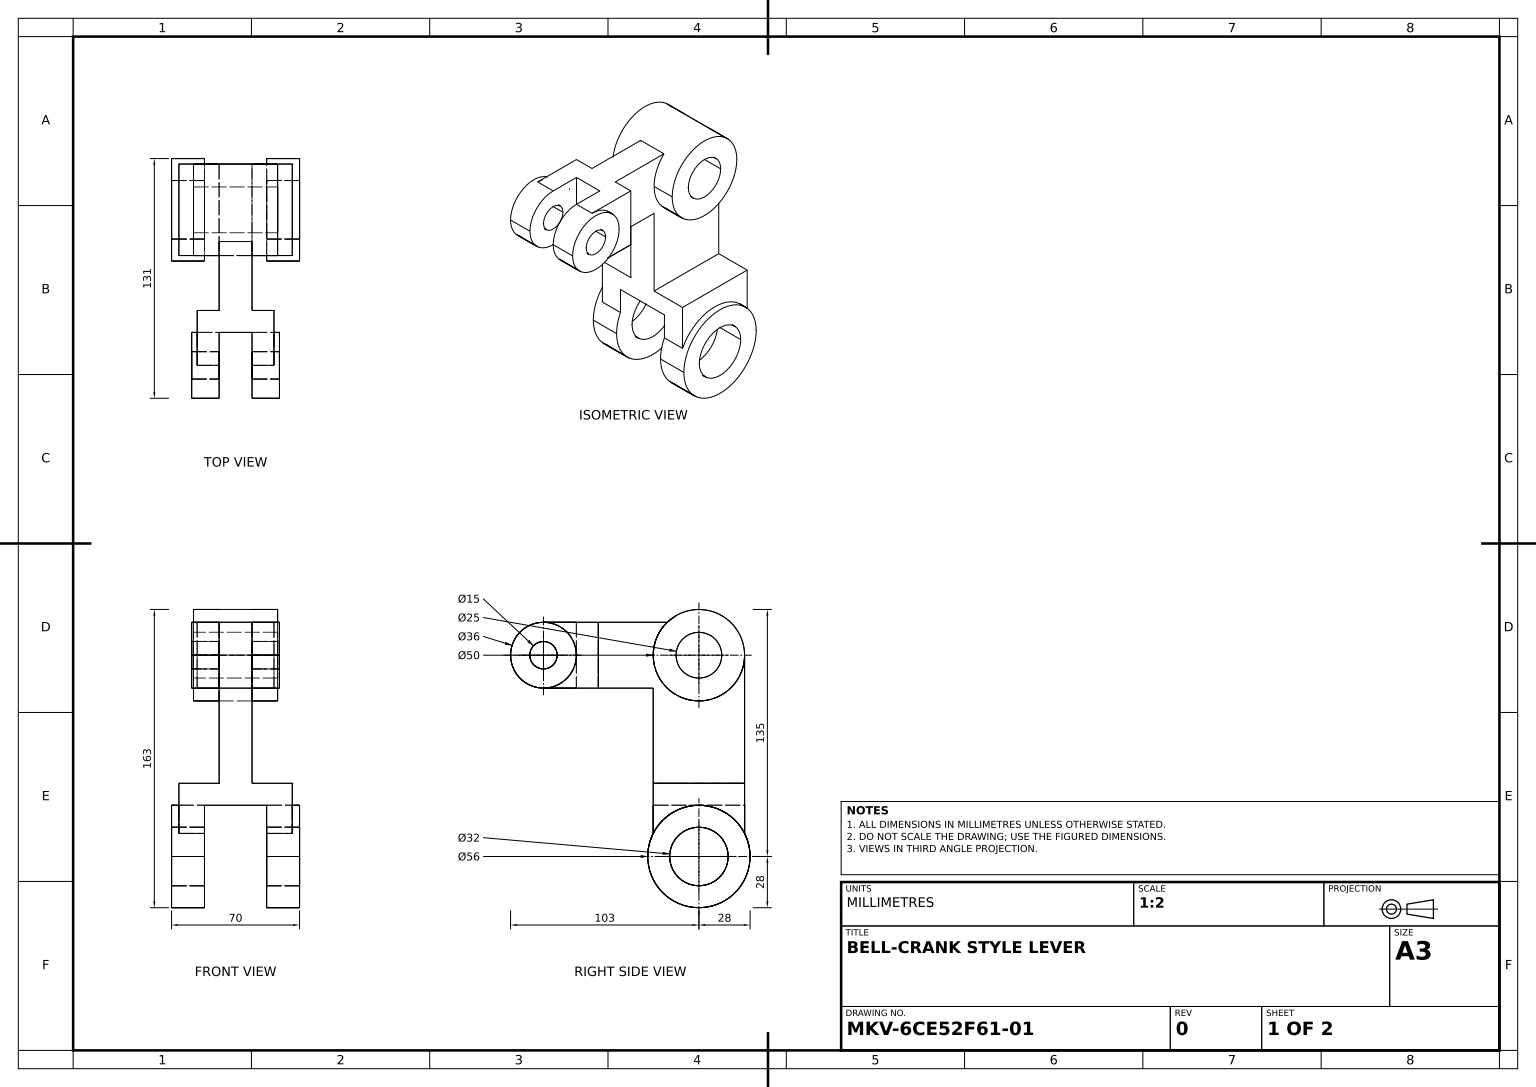
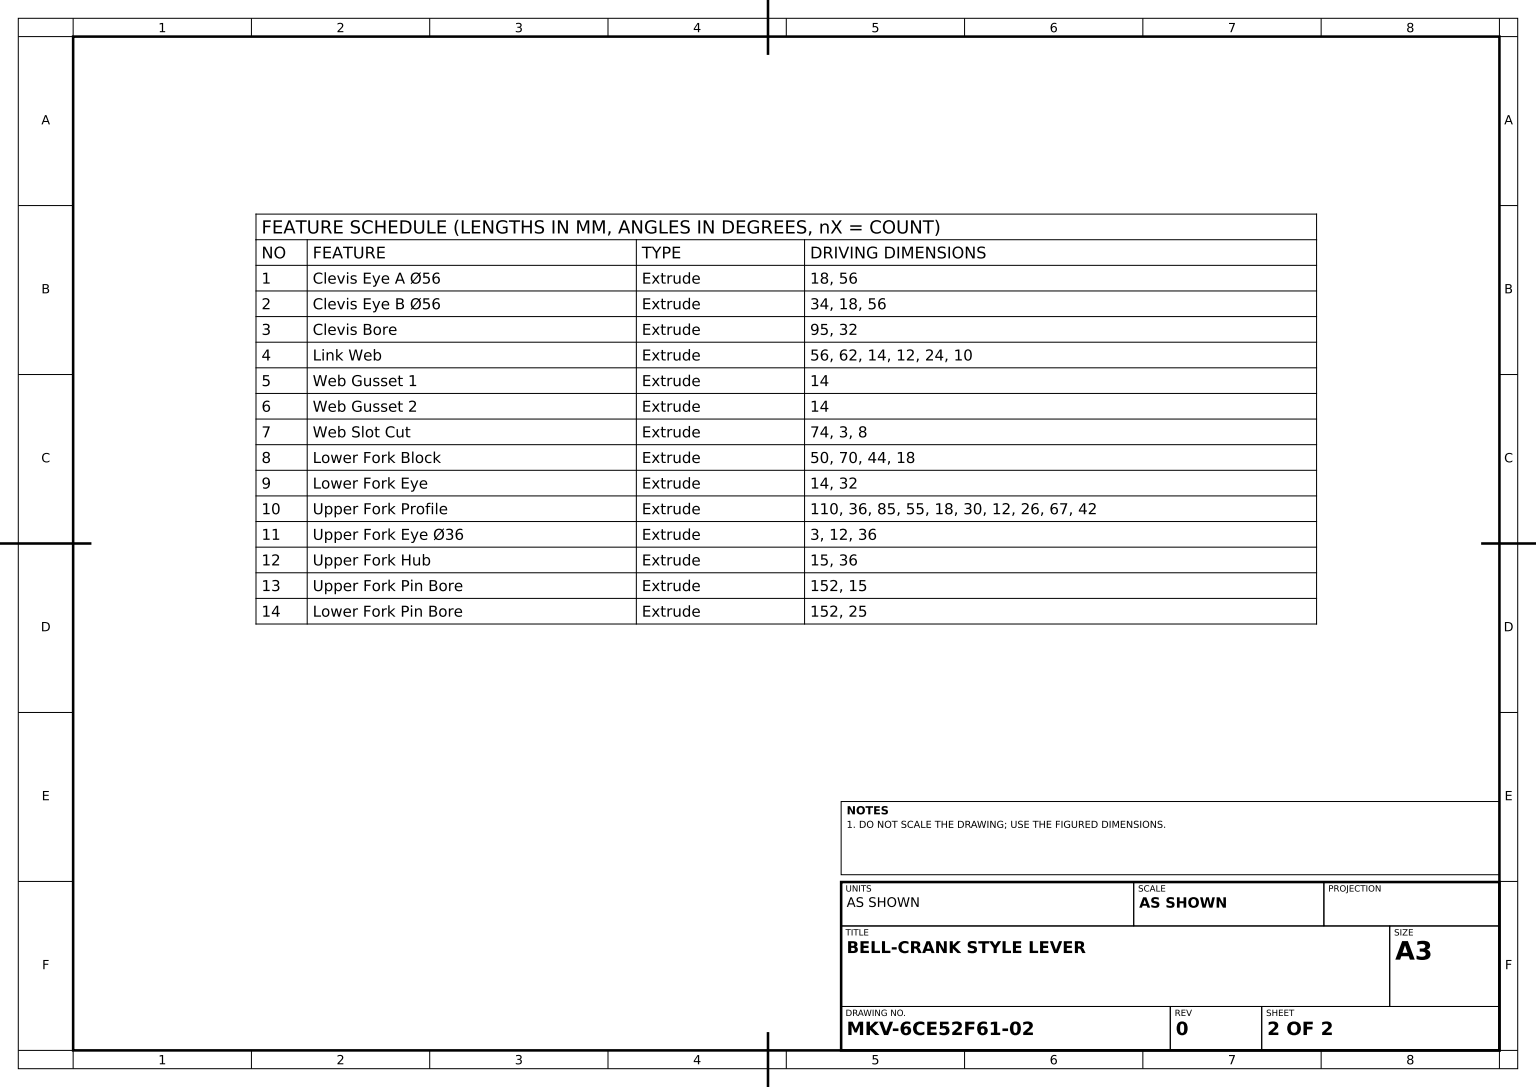
SolidWorks part; units mm, degrees
material "Plain Carbon Steel"
ref_plane "Front Plane" through (0, 0, 0) normal (0, 0, 1) x (1, 0, 0)
ref_plane "Top Plane" through (0, 0, 0) normal (0, 1, 0) x (1, 0, 0)
ref_plane "Right Plane" through (0, 0, 0) normal (1, 0, 0) x (0, 0, -1)
sketch "Clevis Eye A Sketch" plane through (0, 0, 0) normal (1, 0, 0) x (0, 0, -1)
  circle A0 centre (0, 0) radius 28
  dimension "D1" = 56
extrude "Clevis Eye A Ø56" add sketch "Clevis Eye A Sketch" against normal blind 18
ref_plane "Clevis Eye B Plane" through (-52, 0, 0) normal (-1, 0, 0) x (0, 0, 1)
sketch "Clevis Eye B Sketch" plane through (-52, 0, 0) normal (-1, 0, 0) x (0, 0, 1)
  circle A0 centre (0, 0) radius 28
  dimension "D1" = 56
extrude "Clevis Eye B Ø56" add sketch "Clevis Eye B Sketch" along normal blind 18 separate body
sketch "Clevis Bore Sketch" plane through (0, 0, 0) normal (1, 0, 0) x (0, 0, -1)
  circle A0 centre (0, 0) radius 16
  dimension "D1" = 32
extrude "Clevis Bore" cut sketch "Clevis Bore Sketch" against normal blind 95
sketch "Link Web Sketch" plane through (0, 0, 0) normal (0, 0, 1) x (1, 0, 0)
  line L0 (-66, 16) -> (-52, 16)
  line L3 (-4, 40) -> (-66, 40)
  line L6 (-52, -28) -> (-52, 28) construction
  line L7 (-52, 26) -> (-52, 28)
  line L8 (-52, 28) -> (-18, 28)
  line L9 (-18, 28) -> (-18, 26)
  line L10 (-18, 28) -> (-18, -28) construction
  line L12 (-66, 40) -> (-66, 16)
  line L13 (-52, 16) -> (-52, 28)
  line L14 (-4, 40) -> (-4, 16)
  line L15 (-4, 16) -> (-18, 16)
  line L16 (-18, 16) -> (-18, 28)
  dimension "D1" = 62
  dimension "D2" = 14
  dimension "D3" = 12
  dimension "D4" = 24
  dimension "D5" = 10
extrude "Link Web" add sketch "Link Web Sketch" along normal mid plane 56 contours L16 L15 L14 L3 L12 L0 L13 L7 L8 L9
sketch "Web Gusset 1 Sketch" plane through (-4, 0, 0) normal (1, 0, 0) x (0, 0, -1)
  line L0 (-28, 16) -> (-28, 0)
  line L1 (28, 16) -> (28, 0)
  line L2 (-28, 16) -> (-22.9783, 16)
  line L3 (22.9783, 16) -> (28, 16)
  circle A0 centre (0, 0) radius 28 construction
  arc A1 (28, 0) -> (22.9783, 16) centre (0, 0) ccw
  arc A2 (-22.9783, 16) -> (-28, 0) centre (0, 0) ccw
extrude "Web Gusset 1" add sketch "Web Gusset 1 Sketch" against normal blind 14
sketch "Web Gusset 2 Sketch" plane through (-66, 0, 0) normal (-1, 0, 0) x (0, 0, 1)
  line L0 (28, 16) -> (28, 0)
  line L1 (-28, 0) -> (-28, 16)
  line L2 (-28, 16) -> (-22.9783, 16)
  line L3 (28, 16) -> (22.9783, 16)
  circle A0 centre (0, 0) radius 28 construction
  arc A3 (28, 0) -> (22.9783, 16) centre (0, 0) ccw
  arc A4 (-22.9783, 16) -> (-28, 0) centre (0, 0) ccw
extrude "Web Gusset 2" add sketch "Web Gusset 2 Sketch" against normal blind 14
sketch "Web Slot Sketch" plane through (-4, 0, 0) normal (1, 0, 0) x (0, 0, -1)
  line L0 (0, 40) -> (25, 40)
  line L1 (-28, 40) -> (28, 40) construction
  line L2 (25, 40) -> (25, 8)
  line L3 (25, 8) -> (-25, 8)
  line L4 (-25, 8) -> (-25, 40)
  line L5 (-25, 40) -> (0, 40)
  line L6 (25, 40) -> (28, 40)
  line L7 (28, 40) -> (28, 0)
  line L8 (-28, 40) -> (-28, 0)
  line L9 (-28, 40) -> (-28, 0) construction
  arc A0 (28, 0) -> (25, 12.6095) centre (0, 0) ccw
  arc A1 (-25, 12.6095) -> (-28, 0) centre (0, 0) ccw
  line M7 (-28, 40) -> (-28, 0)
  arc M8 (-28, 0) -> (28, 0) centre (0, 0) cw
  line M9 (28, 0) -> (28, 40)
  line M10 (28, 40) -> (-28, 40)
  dimension "D1" = 3
  dimension "D2" = 8
extrude "Web Slot Cut" cut sketch "Web Slot Sketch" against normal blind 74 contours L4 M8 M10 M7 | L2 M10 M8 M9
sketch "Lower Fork Block Sketch" plane through (0, 0, 25) normal (0, 0, 1) x (1, 0, 0)
  line L0 (-44, 40) -> (-26, 40)
  line L1 (-66, 40) -> (-4, 40) construction
  line L2 (-44, 40) -> (-44, 110)
  line L3 (-44, 110) -> (-26, 110)
  line L4 (-26, 110) -> (-26, 40)
  dimension "D1" = 70
  dimension "D2" = 44
  dimension "D3" = 18
extrude "Lower Fork Block" add sketch "Lower Fork Block Sketch" against normal blind 50
sketch "Lower Fork Eye Sketch" plane through (-44, 0, 0) normal (-1, 0, 0) x (0, 0, 1)
  line L0 (-25, 110) -> (25, 110) construction
  circle A0 centre (0, 110) radius 25
extrude "Lower Fork Eye" add sketch "Lower Fork Eye Sketch" along normal blind 14 and the other way blind 32
ref_plane "Fork End Plane" through (0, 110, 0) normal (0, 1, 0) x (1, 0, 0)
sketch "Upper Fork Profile Sketch" plane through (0, 110, 0) normal (0, 1, 0) x (1, 0, 0)
  line L1 (-26, -55) -> (-14, -55)
  line L14 (-26, 0) -> (-26, -55)
  line L16 (-44, -55) -> (-44, 0)
  line L17 (-44, 0) -> (-26, 0)
  line L18 (-14, -55) -> (-14, -85)
  line L19 (-14, -85) -> (-26, -85)
  line L20 (-26, -85) -> (-26, -67)
  line L21 (-26, -67) -> (-44, -67)
  line L22 (-44, -67) -> (-44, -85)
  line L23 (-44, -85) -> (-56, -85)
  line L24 (-56, -85) -> (-56, -55)
  line L25 (-56, -55) -> (-44, -55)
  dimension "D1" = 85
  dimension "D2" = 55
  dimension "D3" = 18
  dimension "D4" = 18
  dimension "D5" = 30
  dimension "D6" = 30
  dimension "D7" = 12
  dimension "D8" = 26
  dimension "D9" = 67
  dimension "D10" = 12
  dimension "D11" = 42
extrude "Upper Fork Profile" add sketch "Upper Fork Profile Sketch" along normal mid plane 36
sketch "Upper Fork Eye Sketch Ø36" plane through (-14, 0, 0) normal (1, 0, 0) x (0, 0, -1)
  line L0 (-85, 128) -> (-85, 92) construction
  circle A0 centre (-85, 110) radius 18
  dimension "D1" = 36
extrude "Upper Fork Eye Ø36" add sketch "Upper Fork Eye Sketch Ø36" along normal blind 3 and the other way blind 12
sketch "Upper Fork Hub Sketch" plane through (-44, 0, 0) normal (1, 0, 0) x (0, 0, -1)
  circle A0 centre (-85, 110) radius 18
  dimension "D1" = 36
extrude "Upper Fork Hub" add sketch "Upper Fork Hub Sketch" against normal blind 15
sketch "Upper Fork Pin Bore Sketch" plane through (-11, 0, 0) normal (1, 0, 0) x (0, 0, -1)
  circle A0 centre (-85, 110) radius 7.5
  dimension "D1" = 15
extrude "Upper Fork Pin Bore" cut sketch "Upper Fork Pin Bore Sketch" against normal blind 152
sketch "Lower Fork Pin Bore Sketch" plane through (-12, 0, 0) normal (1, 0, 0) x (0, 0, -1)
  circle A0 centre (0, 110) radius 12.5
  dimension "D1" = 25
extrude "Lower Fork Pin Bore" cut sketch "Lower Fork Pin Bore Sketch" against normal blind 152
